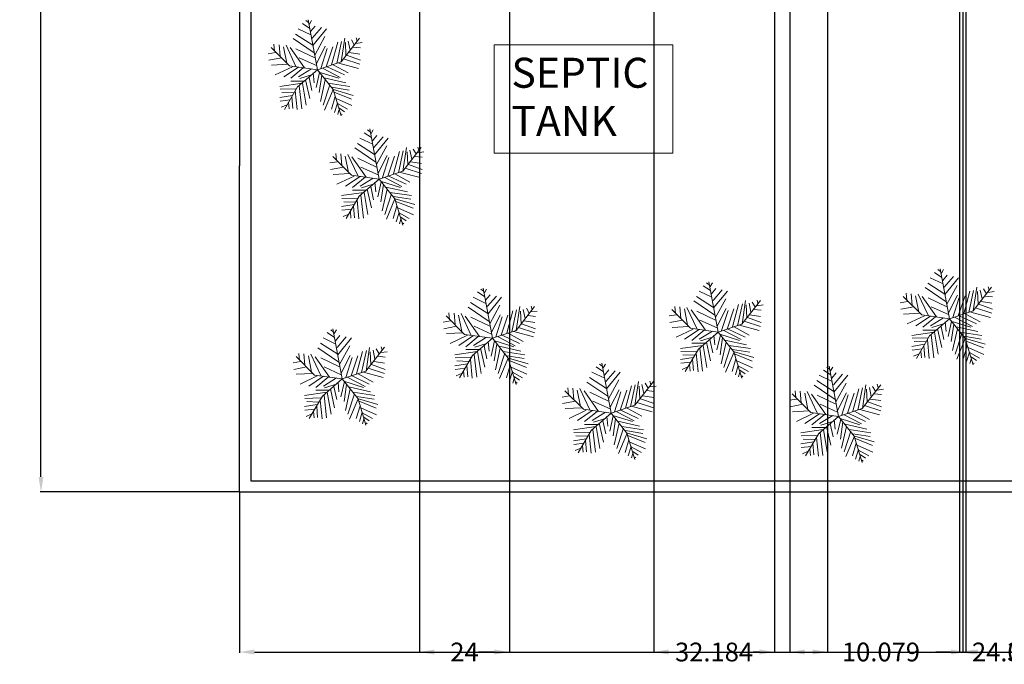
# Model space of a CAD drawing. Units: inches. Extents: x 460 to 1030, y -658 to 271.
# Tile 1 of 10: x 465 to 728, y -658 to -486. Entities that reach past the tile are written whole.
import ezdxf

# ---------------------------------------------------------------- set-up
doc = ezdxf.new("R2010")
doc.units = ezdxf.units.IN
doc.header["$MEASUREMENT"] = 0
for name, color, linetype, lineweight in [('A-ANNO-DIMS', 2, 'Continuous', 18), ('C-ANNO-TEXT', 7, 'Continuous', 18), ('C-PROP', 7, 'Continuous', 25), ('C-UTIL', 8, 'Continuous', 18), ('L-PLNT', 94, 'Continuous', 13)]:
    doc.layers.add(name, color=color, linetype=linetype, lineweight=lineweight)
doc.styles.get("Standard").update_dxf_attribs({"font": 'arial.ttf'})
doc.dimstyles.get("Standard").update_dxf_attribs({"dimtxt": 5, "dimasz": 4, "dimexe": 0.18, "dimexo": 0.0625, "dimgap": 0.09, "dimtad": 0, "dimtih": 1, "dimtoh": 1, "dimdec": 1, "dimzin": 0, "dimdsep": 46, "dimlunit": 4, "dimtxsty": 'Standard', "dimcen": 0.09, "dimadec": 0, "dimazin": 0, "dimtfac": 1, "dimtdec": 1, "dimtofl": 0, "dimtmove": 0, "dimatfit": 3, "dimfxl": 1, "dimtolj": 1, "dimtzin": 0, "dimarcsym": 0})

# ---------------------------------------------------------------- blocks, each defined once
blk = doc.blocks.new('*U11')
for p, q in [((0, 0), (-266.7, 1447.8)), ((-185.1152, 1008.5578), (-553.1612, 1185.4942)), ((-221.9198, 1197.3052), (-433.5526, 1338.8594)), ((-258.7244, 1362.456), (-332.3336, 1421.4348)), ((-231.1146, 1315.2628), (-166.7002, 1421.4348)), ((-194.31, 1102.9442), (-65.4812, 1256.284)), ((-148.3106, 914.1968), (118.5418, 1220.9018)), ((-129.8956, 701.8528), (265.7602, 1185.4942)), ((-93.091, 489.5342), (-700.3796, 902.3858)), ((-129.8956, 713.6638), (-626.7704, 1032.1544)), ((-74.7014, 418.7444), (219.7608, 961.39)), ((685.8, 228.6), (1219.2, 914.4)), ((689.0258, 230.0224), (790.2448, 914.1968)), ((983.4626, 867.0036), (1066.2666, 725.4494)), ((1121.4862, 925.9824), (1149.0706, 831.6214)), ((-800.1, 114.3), (-1333.5, 647.7)), ((-1234.059, 536.7274), (-1252.4486, 737.2604)), ((-1105.2302, 725.4494), (-1077.6458, 395.1732)), ((-976.4268, 666.4706), (-884.4026, 194.6402)), ((-902.8176, 713.6638), (-617.5756, 100.2538)), ((-369.1382, 53.086), (-783.1836, 642.874)), ((-617.5756, 607.4918), (-74.7014, 347.98)), ((-28.6766, 171.0436), (228.9556, 678.2816)), ((100.1268, 41.275), (284.1498, 619.2774)), ((256.5654, 88.4682), (449.7832, 666.4706)), ((412.9786, 147.447), (587.8068, 796.2392)), ((560.197, 182.8292), (698.2206, 819.8358)), ((808.6344, 784.4282), (827.0494, 418.7444)), ((891.4384, 831.6214), (946.658, 572.1096)), ((1029.462, 654.685), (1241.0948, 631.0884)), ((1112.2914, 760.8316), (1296.3144, 784.4282)), ((-1206.4492, 501.3198), (-1418.082, 465.9376)), ((-1031.621, 347.98), (-1399.667, 277.1902)), ((-525.5514, 347.98), (-28.6766, 123.8504)), ((753.4148, 312.5978), (1222.6798, 159.2326)), ((845.439, 418.7444), (1241.0948, 277.1902)), ((919.0482, 501.3198), (1222.6798, 454.152)), ((-847.598, 159.2326), (-1326.0578, 135.636)), ((-718.7946, 88.4682), (-1215.644, -147.447)), ((-543.9664, 76.6572), (-967.2066, -206.4512)), ((0, 0), (-800.1, 114.3)), ((-405.9428, 53.086), (-764.794, -241.8334)), ((0, 0), (-571.5, -495.3)), ((-166.7002, 29.4894), (-543.9664, -206.4512)), ((0, 0), (685.8, 228.6)), ((0, 0), (457.2, -571.5)), ((164.5412, 41.275), (661.416, -218.2368)), ((284.1498, 88.4682), (781.0246, -147.447)), ((458.978, 147.447), (891.4384, -88.4682)), ((615.4166, 194.6402), (1185.8752, 41.275)), ((-166.7002, -147.447), (-507.1618, -253.619)), ((-240.3094, -218.2368), (-157.5054, -595.7062)), ((-120.7008, -88.4682), (-93.091, -371.5766)), ((63.3222, -76.6826), (-37.8714, -513.1308)), ((44.9326, -64.897), (615.4166, -241.8334)), ((127.7366, -159.258), (54.1274, -654.685)), ((192.151, -230.0224), (817.8292, -371.5766)), ((-442.7474, -383.3876), (-1086.8406, -477.7486)), ((-617.5756, -548.5384), (-1077.6458, -560.324)), ((-571.5, -495.3), (-952.5, -1143)), ((-387.5278, -324.4088), (-764.794, -324.4088)), ((-525.5514, -465.963), (-451.9422, -1126.5408)), ((-433.5526, -383.3876), (-323.1134, -1020.3688)), ((-341.5284, -289.0012), (-221.9198, -831.6214)), ((228.9556, -289.0012), (90.932, -914.1968)), ((357.759, -430.5554), (164.5412, -1020.3688)), ((311.7596, -383.3876), (937.4378, -477.7486)), ((412.9786, -501.3452), (919.0482, -583.9206)), ((-718.7946, -737.2604), (-1086.8406, -796.2392)), ((-681.9646, -666.496), (-1022.4262, -654.685)), ((-737.1842, -784.4536), (-709.5744, -1114.7298)), ((-635.9652, -607.5172), (-580.771, -1150.1374)), ((458.978, -572.1096), (210.5406, -1161.923)), ((514.1976, -772.6426), (403.7838, -1138.3264)), ((457.2, -571.5), (685.8, -1333.5)), ((468.1982, -572.1096), (1029.462, -737.2604)), ((486.5878, -642.8994), (983.4626, -843.4324)), ((541.8074, -831.6214), (992.6574, -1032.1544)), ((-783.1836, -867.029), (-1077.6458, -902.4112)), ((-875.2078, -1008.5832), (-1040.8412, -1079.3476)), ((-829.2084, -937.7934), (-810.7934, -1126.5408)), ((578.612, -961.39), (495.7826, -1232.7128)), ((578.612, -973.1756), (873.0488, -1138.3264)), ((624.6114, -1102.9442), (781.0246, -1209.1162)), ((624.6114, -1161.923), (587.8068, -1291.6916)), ((679.8056, -1268.095), (716.6102, -1291.6916))]:
    blk.add_line(p, q)
blk = doc.blocks.new('*D39')
at = {"layer": 'A-ANNO-DIMS', "color": 0, "lineweight": -2, "transparency": 16777216}
for p, q in [((523.8, -611.79), (523.8, -654.61)), ((979.8, -611.79), (979.8, -654.61)), ((527.8, -654.43), (746.08, -654.43)), ((975.8, -654.43), (757.51, -654.43))]:
    blk.add_line(p, q, dxfattribs=at)
at = {"layer": 'A-ANNO-DIMS', "color": 0, "transparency": 16777216}
for points in [[(527.8, -653.77), (527.8, -655.1), (523.8, -654.43)], [(975.8, -653.77), (975.8, -655.1), (979.8, -654.43)]]:
    blk.add_solid(points, dxfattribs=at)
at = {"layer": 'Defpoints', "color": 0, "transparency": 16777216}
for p in [(523.8, -611.73), (979.8, -611.73), (979.8, -654.43)]:
    blk.add_point(p, dxfattribs=at)
at = {"layer": 'A-ANNO-DIMS', "color": 0, "transparency": 16777216, "insert": (751.8, -654.43), "char_height": 5, "attachment_point": 5}
blk.add_mtext('\\A1;456', dxfattribs=at)
blk = doc.blocks.new('*D40')
at = {"layer": 'A-ANNO-DIMS', "color": 0, "lineweight": -2, "transparency": 16777216}
for p, q in [((523.73, 201.27), (470.68, 201.27)), ((470.86, 197.27), (470.86, -202.58)), ((470.86, -607.73), (470.86, -207.87)), ((523.73, -611.73), (470.68, -611.73))]:
    blk.add_line(p, q, dxfattribs=at)
at = {"layer": 'A-ANNO-DIMS', "color": 0, "transparency": 16777216}
for points in [[(470.19, 197.27), (471.52, 197.27), (470.86, 201.27)], [(470.19, -607.73), (471.52, -607.73), (470.86, -611.73)]]:
    blk.add_solid(points, dxfattribs=at)
at = {"layer": 'Defpoints', "color": 0, "transparency": 16777216}
for p in [(470.86, 201.27), (523.8, 201.27), (523.8, -611.73)]:
    blk.add_point(p, dxfattribs=at)
at = {"layer": 'A-ANNO-DIMS', "color": 0, "transparency": 16777216, "insert": (470.86, -205.23), "char_height": 5, "attachment_point": 5}
blk.add_mtext('\\A1;813', dxfattribs=at)
blk = doc.blocks.new('*D51')
at = {"layer": 'A-ANNO-DIMS', "color": 0, "lineweight": -2, "transparency": 16777216}
for p, q in [((670.56, -476.79), (670.56, -654.61)), ((680.64, -476.79), (680.64, -654.61)), ((674.56, -654.43), (676.64, -654.43)), ((680.64, -654.43), (684.64, -654.43))]:
    blk.add_line(p, q, dxfattribs=at)
at = {"layer": 'A-ANNO-DIMS', "color": 0, "transparency": 16777216}
for points in [[(674.56, -653.77), (674.56, -655.1), (670.56, -654.43)], [(676.64, -653.77), (676.64, -655.1), (680.64, -654.43)]]:
    blk.add_solid(points, dxfattribs=at)
at = {"layer": 'Defpoints', "color": 0, "transparency": 16777216}
for p in [(670.56, -476.73), (680.64, -476.73), (680.64, -654.43)]:
    blk.add_point(p, dxfattribs=at)
at = {"layer": 'A-ANNO-DIMS', "color": 0, "transparency": 16777216, "insert": (694.88, -654.43), "char_height": 5, "attachment_point": 5}
blk.add_mtext('\\A1;10.079', dxfattribs=at)
blk = doc.blocks.new('*D57')
at = {"layer": 'A-ANNO-DIMS', "color": 0, "lineweight": -2, "transparency": 16777216}
for p, q in [((717.53, -38.79), (717.53, -654.61)), ((741.59, -38.79), (741.59, -654.61)), ((713.53, -654.43), (709.53, -654.43)), ((745.59, -654.43), (749.59, -654.43))]:
    blk.add_line(p, q, dxfattribs=at)
at = {"layer": 'A-ANNO-DIMS', "color": 0, "transparency": 16777216}
for points in [[(713.53, -653.77), (713.53, -655.1), (717.53, -654.43)], [(745.59, -653.77), (745.59, -655.1), (741.59, -654.43)]]:
    blk.add_solid(points, dxfattribs=at)
at = {"layer": 'Defpoints', "color": 0, "transparency": 16777216}
for p in [(717.53, -38.73), (741.59, -38.73), (741.59, -654.43)]:
    blk.add_point(p, dxfattribs=at)
at = {"layer": 'A-ANNO-DIMS', "color": 0, "transparency": 16777216, "insert": (729.56, -654.43), "char_height": 5, "attachment_point": 5}
blk.add_mtext('\\A1;24.065', dxfattribs=at)
blk = doc.blocks.new('*D63')
at = {"layer": 'A-ANNO-DIMS', "color": 0, "lineweight": -2, "transparency": 16777216}
for p, q in [((571.8, -281.79), (571.8, -654.61)), ((595.8, -281.79), (595.8, -654.61)), ((575.8, -654.43), (580.09, -654.43)), ((591.8, -654.43), (587.5, -654.43))]:
    blk.add_line(p, q, dxfattribs=at)
at = {"layer": 'A-ANNO-DIMS', "color": 0, "transparency": 16777216}
for points in [[(575.8, -653.77), (575.8, -655.1), (571.8, -654.43)], [(591.8, -653.77), (591.8, -655.1), (595.8, -654.43)]]:
    blk.add_solid(points, dxfattribs=at)
at = {"layer": 'Defpoints', "color": 0, "transparency": 16777216}
for p in [(571.8, -281.73), (595.8, -281.73), (595.8, -654.43)]:
    blk.add_point(p, dxfattribs=at)
at = {"layer": 'A-ANNO-DIMS', "color": 0, "transparency": 16777216, "insert": (583.8, -654.43), "char_height": 5, "attachment_point": 5}
blk.add_mtext('\\A1;24', dxfattribs=at)
blk = doc.blocks.new('*D68')
at = {"layer": 'A-ANNO-DIMS', "color": 0, "lineweight": -2, "transparency": 16777216}
for p, q in [((634.27, 90.21), (634.27, -654.61)), ((666.46, 90.21), (666.46, -654.61)), ((638.27, -654.43), (639.91, -654.43)), ((662.46, -654.43), (660.82, -654.43))]:
    blk.add_line(p, q, dxfattribs=at)
at = {"layer": 'A-ANNO-DIMS', "color": 0, "transparency": 16777216}
for points in [[(638.27, -653.77), (638.27, -655.1), (634.27, -654.43)], [(662.46, -653.77), (662.46, -655.1), (666.46, -654.43)]]:
    blk.add_solid(points, dxfattribs=at)
at = {"layer": 'Defpoints', "color": 0, "transparency": 16777216}
for p in [(634.27, 90.27), (666.46, 90.27), (666.46, -654.43)]:
    blk.add_point(p, dxfattribs=at)
at = {"layer": 'A-ANNO-DIMS', "color": 0, "transparency": 16777216, "insert": (650.37, -654.43), "char_height": 5, "attachment_point": 5}
blk.add_mtext('\\A1;32.184', dxfattribs=at)
blk = doc.blocks.new('*D70')
at = {"layer": 'A-ANNO-DIMS', "color": 0, "lineweight": -2, "transparency": 16777216}
for p, q in [((716.71, -287.79), (716.71, -654.61)), ((789.82, -287.79), (789.82, -654.61)), ((720.71, -654.43), (744.79, -654.43)), ((785.82, -654.43), (761.75, -654.43))]:
    blk.add_line(p, q, dxfattribs=at)
at = {"layer": 'A-ANNO-DIMS', "color": 0, "transparency": 16777216}
for points in [[(720.71, -653.77), (720.71, -655.1), (716.71, -654.43)], [(785.82, -653.77), (785.82, -655.1), (789.82, -654.43)]]:
    blk.add_solid(points, dxfattribs=at)
at = {"layer": 'Defpoints', "color": 0, "transparency": 16777216}
for p in [(716.71, -287.73), (789.82, -287.73), (789.82, -654.43)]:
    blk.add_point(p, dxfattribs=at)
at = {"layer": 'A-ANNO-DIMS', "color": 0, "transparency": 16777216, "insert": (753.27, -654.43), "char_height": 5, "attachment_point": 5}
blk.add_mtext('\\A1;73.12', dxfattribs=at)
blk = doc.blocks.new('*D72')
at = {"layer": 'A-ANNO-DIMS', "color": 0, "lineweight": -2, "transparency": 16777216}
for p, q in [((715.8, 68.25), (715.8, -654.61)), ((748.8, 57.75), (748.8, -654.61)), ((719.8, -654.43), (728.63, -654.43)), ((744.8, -654.43), (735.97, -654.43))]:
    blk.add_line(p, q, dxfattribs=at)
at = {"layer": 'A-ANNO-DIMS', "color": 0, "transparency": 16777216}
for points in [[(719.8, -653.77), (719.8, -655.1), (715.8, -654.43)], [(744.8, -653.77), (744.8, -655.1), (748.8, -654.43)]]:
    blk.add_solid(points, dxfattribs=at)
at = {"layer": 'Defpoints', "color": 0, "transparency": 16777216}
for p in [(715.8, 68.31), (748.8, 57.81), (748.8, -654.43)]:
    blk.add_point(p, dxfattribs=at)
at = {"layer": 'A-ANNO-DIMS', "color": 0, "transparency": 16777216, "insert": (732.3, -654.43), "char_height": 5, "attachment_point": 5}
blk.add_mtext('\\A1;33', dxfattribs=at)

msp = doc.modelspace()

# ---------------------------------------------------------------- linework, layer by layer
at = {"layer": 'C-PROP'}
for p, q in [((523.7961, 129.2738), (523.7961, -524.7262)), ((526.7961, 126.2738), (526.7961, -608.7262)), ((523.7961, -611.7262), (523.7961, -524.7262)), ((526.7961, -608.7262), (799.8801, -608.7262)), ((523.7961, -611.7262), (979.7961, -611.7262)), ((582.931, -611.7262), (582.931, -611.7262))]:
    msp.add_line(p, q, dxfattribs=at)
at = {"layer": 'C-UTIL'}
msp.add_lwpolyline([(591.7361, -492.3933), (639.3933, -492.3933), (639.3933, -521.3431), (591.7361, -521.3431)], close=True, dxfattribs=at)

# ---------------------------------------------------------------- block references
at = {"layer": 'L-PLNT', "xscale": 0.0092368434635362, "yscale": 0.0092368434635362, "zscale": 0.0092368434635362}
for p in [(544.5653, -499.1011), (561.027, -528.2553), (713.1416, -565.5309), (651.4622, -569.0711), (591.2416, -570.737), (551.1931, -581.5884), (622.9147, -590.7285), (683.5522, -591.5615)]:
    msp.add_blockref('*U11', p, dxfattribs=at)

# ---------------------------------------------------------------- texts
at = {"layer": 'C-ANNO-TEXT'}
for s, p in [('SEPTIC ', (596.3332, -503.8872)), ('TANK', (596.3332, -516.7385))]:
    msp.add_text(s, height=8, dxfattribs=at).set_placement(p)

# ---------------------------------------------------------------- dimensions: what is measured, and where the dimension line sits
at = {"layer": 'A-ANNO-DIMS'}
dim = msp.add_linear_dim(base=(470.8563, 201.2738), p1=(523.7961, -611.7262), p2=(523.7961, 201.2738), angle=90, dimstyle='Standard', override={"dimdec": 0, "dimlfac": 1, "dimrnd": 0, "dimzin": 0, "dimdsep": 46, "dimlunit": 2}, dxfattribs=at)
dim.commit()
dim.dimension.update_dxf_attribs({"geometry": '*D40', "text_midpoint": (470.8563, -205.2262)})
for base, p1, p2, override, picture, middle in [((666.4584, -654.4339), (634.2742, 90.2738), (666.4584, 90.2738), {"dimdec": 3, "dimlfac": 1, "dimrnd": 0, "dimzin": 0, "dimdsep": 46, "dimlunit": 2}, '*D68', (650.3663, -654.4339)), ((748.7961, -654.4339), (715.7961, 68.3148), (748.7961, 57.8148), {"dimdec": 0, "dimlfac": 1, "dimrnd": 0, "dimzin": 0, "dimdsep": 46, "dimlunit": 2}, '*D72', (732.2961, -654.4339)), ((741.5908, -654.4339), (717.5258, -38.7262), (741.5908, -38.7262), {"dimdec": 3, "dimlfac": 1, "dimrnd": 0, "dimzin": 0, "dimdsep": 46, "dimlunit": 2}, '*D57', (729.5583, -654.4339)), ((595.7961, -654.4339), (571.7961, -281.7262), (595.7961, -281.7262), {"dimdec": 0, "dimlfac": 1, "dimrnd": 0, "dimzin": 0, "dimdsep": 46, "dimlunit": 2}, '*D63', (583.7961, -654.4339)), ((789.8237, -654.4339), (716.7073, -287.7262), (789.8237, -287.7262), {"dimdec": 2, "dimlfac": 1, "dimrnd": 0, "dimzin": 0, "dimdsep": 46, "dimlunit": 2}, '*D70', (753.2655, -654.4339)), ((680.6383, -654.4339), (670.5594, -476.7262), (680.6383, -476.7262), {"dimdec": 3, "dimlfac": 1, "dimrnd": 0, "dimzin": 0, "dimdsep": 46, "dimlunit": 2}, '*D51', (694.8767, -654.4339)), ((979.7961, -654.4339), (523.7961, -611.7262), (979.7961, -611.7262), {"dimdec": 0, "dimlfac": 1, "dimrnd": 0, "dimzin": 0, "dimdsep": 46, "dimlunit": 2}, '*D39', (751.7961, -654.4339))]:
    dim = msp.add_linear_dim(base=base, p1=p1, p2=p2, dimstyle='Standard', override=override, dxfattribs=at)
    dim.commit()
    dim.dimension.update_dxf_attribs({"geometry": picture, "text_midpoint": middle})

doc.saveas('drawing.dxf')
